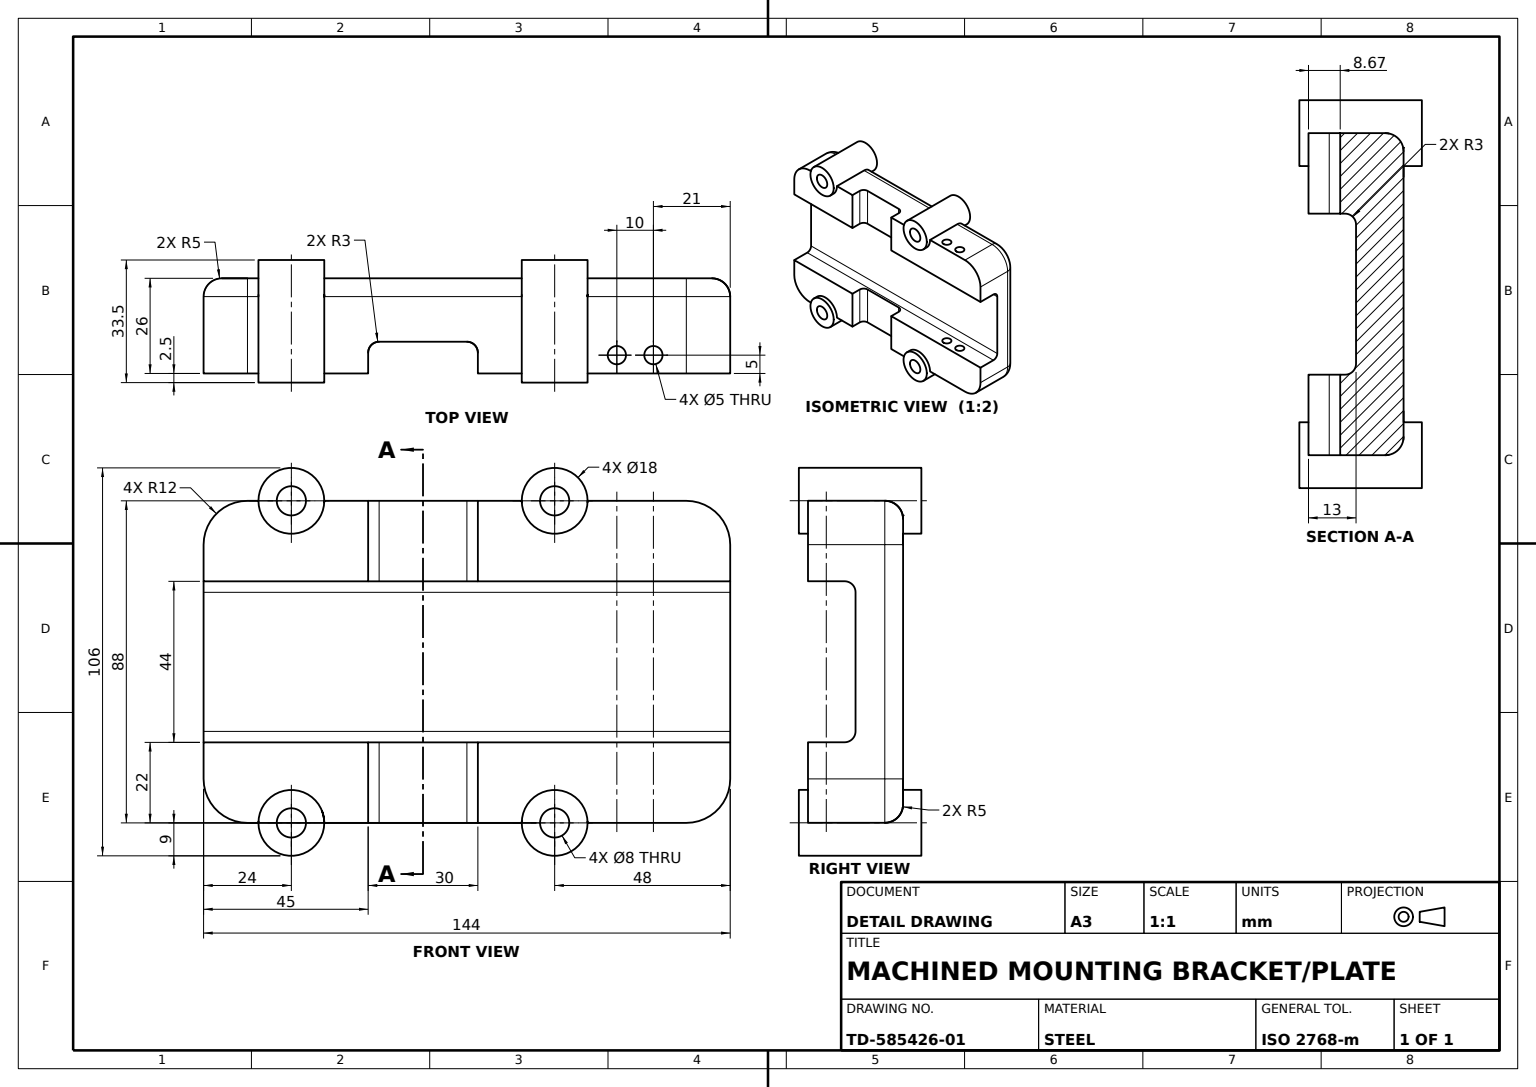
from build123d import *

# Parameters (mm, degrees)
BASE_PLATE_SKETCH_W                      = 144
BASE_PLATE_SKETCH_H                      = 88
BASE_PLATE_144X88_DEPTH                  = 26
PLATE_CORNER_FILLETS_R12_R               = 12
PLATE_EDGE_FILLETS_R5_R                  = 5
CORNER_BOSSES_DEPTH                      = 28.5
CORNER_BOSSES_DEPTH_BACK                 = 5
CORNER_BOSS_SKETCH_R                     = 9
CORNER_BOSS_SKETCH_R_2                   = 4
CORNER_BOSS_HOLES_DEPTH                  = 94.836293705
CORNER_BOSS_HOLES_DEPTH_BACK             = 94.836293705
SKETCH3_2_R                              = 4
CENTER_CHANNEL_CUT_DEPTH                 = 94.836293705
CENTER_CHANNEL_CUT_DEPTH_BACK            = 94.836293705
SIDE_RAIL_SLOTS_AND_PIN_HOLES_DEPTH      = 94.836293705
SIDE_RAIL_SLOTS_AND_PIN_HOLES_DEPTH_BACK = 94.836293705
SIDE_RAIL_SLOT_SKETCH_R                  = 2.5


with BuildPart() as part:
    # Base Plate Sketch → Base Plate 144x88 (new body)
    with BuildSketch(Plane.XY):
        Rectangle(BASE_PLATE_SKETCH_W, BASE_PLATE_SKETCH_H)
    extrude(amount=BASE_PLATE_144X88_DEPTH)

    # Plate Corner Fillets R12
    plate_corner_fillets_r12_edges = [part.edges().sort_by_distance(p)[0] for p in [
        (72, -44, 13),
        (-72, -44, 13),
        (-72, 44, 13),
        (72, 44, 13),
    ]]
    fillet(plate_corner_fillets_r12_edges, radius=PLATE_CORNER_FILLETS_R12_R)

    # Plate Edge Fillets R5
    plate_edge_fillets_r5_edges = [part.edges().sort_by_distance(p)[0] for p in [
        (72, 0, 0),
        (0, -44, 0),
        (-72, 0, 0),
        (0, 44, 0),
        (68.485281374, 40.485281374, 0),
        (-68.485281374, 40.485281374, 0),
        (-68.485281374, -40.485281374, 0),
        (68.485281374, -40.485281374, 0),
    ]]
    fillet(plate_edge_fillets_r5_edges, radius=PLATE_EDGE_FILLETS_R5_R)

    # Corner Boss Sketch → Corner Bosses (add, two sides: drawn at the far end of the back side and taken through both)
    # profile 1 of 4: a face of its own
    with BuildSketch(Plane.XY.offset(-CORNER_BOSSES_DEPTH_BACK)):
        with Locations((24, 44)):
            Circle(CORNER_BOSS_SKETCH_R)
        with Locations((24, 44)):
            Circle(CORNER_BOSS_SKETCH_R_2, mode=Mode.SUBTRACT)
    # profile 2 of 4: a face of its own
    with BuildSketch(Plane.XY.offset(-CORNER_BOSSES_DEPTH_BACK)):
        with Locations((-48, 44)):
            Circle(CORNER_BOSS_SKETCH_R)
        with Locations((-48, 44)):
            Circle(CORNER_BOSS_SKETCH_R_2, mode=Mode.SUBTRACT)
    # profile 3 of 4: a face of its own
    with BuildSketch(Plane.XY.offset(-CORNER_BOSSES_DEPTH_BACK)):
        with Locations((-48, -44)):
            Circle(CORNER_BOSS_SKETCH_R)
        with Locations((-48, -44)):
            Circle(CORNER_BOSS_SKETCH_R_2, mode=Mode.SUBTRACT)
    # profile 4 of 4: a face of its own
    with BuildSketch(Plane.XY.offset(-CORNER_BOSSES_DEPTH_BACK)):
        with Locations((24, -44)):
            Circle(CORNER_BOSS_SKETCH_R)
        with Locations((24, -44)):
            Circle(CORNER_BOSS_SKETCH_R_2, mode=Mode.SUBTRACT)
    extrude(amount=CORNER_BOSSES_DEPTH + CORNER_BOSSES_DEPTH_BACK)

    # Sketch3_2 → Corner Boss Holes (cut, two sides: drawn at the far end of the back side and taken through both)
    with BuildSketch(Plane.XY.offset(-CORNER_BOSS_HOLES_DEPTH_BACK)):
        with Locations(Location((24, 44, 0), (0, 0, 180))):
            Circle(SKETCH3_2_R)
        with Locations(Location((-48, 44, 0), (0, 0, 180))):
            Circle(SKETCH3_2_R)
        with Locations(Location((-48, -44, 0), (0, 0, 180))):
            Circle(SKETCH3_2_R)
        with Locations(Location((24, -44, 0), (0, 0, 180))):
            Circle(SKETCH3_2_R)
    extrude(amount=CORNER_BOSS_HOLES_DEPTH + CORNER_BOSS_HOLES_DEPTH_BACK, mode=Mode.SUBTRACT)


with BuildPart() as corner_boss_holes_kept_piece:
    # of the separate pieces the step leaves, the one the design keeps (corner_boss_holes_pieces_kept)
    add(part.part.solids().sort_by_distance((60, 39, 0))[0])

    # Center Channel Sketch → Center Channel Cut (cut, two sides: drawn at the far end of the back side and taken through both)
    with BuildSketch(Plane(origin=(0, 0, 0), x_dir=(0, 0, -1), z_dir=(1, 0, 0)).offset(-CENTER_CHANNEL_CUT_DEPTH_BACK)):
        with BuildLine():
            Line((-26, 22), (-16, 22))
            ThreePointArc((-16, 22), (-13.878679656, 21.121320344), (-13, 19))
            Line((-13, 19), (-13, -19))
            ThreePointArc((-13, -19), (-13.878679656, -21.121320344), (-16, -22))
            Line((-16, -22), (-26, -22))
            Line((-26, -22), (-26, 22))
        make_face()
    extrude(amount=CENTER_CHANNEL_CUT_DEPTH + CENTER_CHANNEL_CUT_DEPTH_BACK, mode=Mode.SUBTRACT)

    # Side Rail Slot Sketch → Side Rail Slots and Pin Holes (cut, two sides: drawn at the far end of the back side and taken through both)
    with BuildSketch(Plane(origin=(0, 0, 0), x_dir=(1, 0, 0), z_dir=(0, 1, 0)).offset(-SIDE_RAIL_SLOTS_AND_PIN_HOLES_DEPTH_BACK)):
        with Locations(Location((51, -21, 0), (0, 0, 270))):
            Circle(SIDE_RAIL_SLOT_SKETCH_R)
        with Locations(Location((41, -21, 0), (0, 0, 270))):
            Circle(SIDE_RAIL_SLOT_SKETCH_R)
        with BuildLine():
            Line((-27, -26), (3, -26))
            Line((3, -26), (3, -20.33))
            ThreePointArc((3, -20.33), (2.121320344, -18.208679656), (0, -17.33))
            Line((0, -17.33), (-24, -17.33))
            ThreePointArc((-24, -17.33), (-26.121320344, -18.208679656), (-27, -20.33))
            Line((-27, -20.33), (-27, -26))
        make_face()
    extrude(amount=SIDE_RAIL_SLOTS_AND_PIN_HOLES_DEPTH + SIDE_RAIL_SLOTS_AND_PIN_HOLES_DEPTH_BACK, mode=Mode.SUBTRACT)


solid = corner_boss_holes_kept_piece.part
